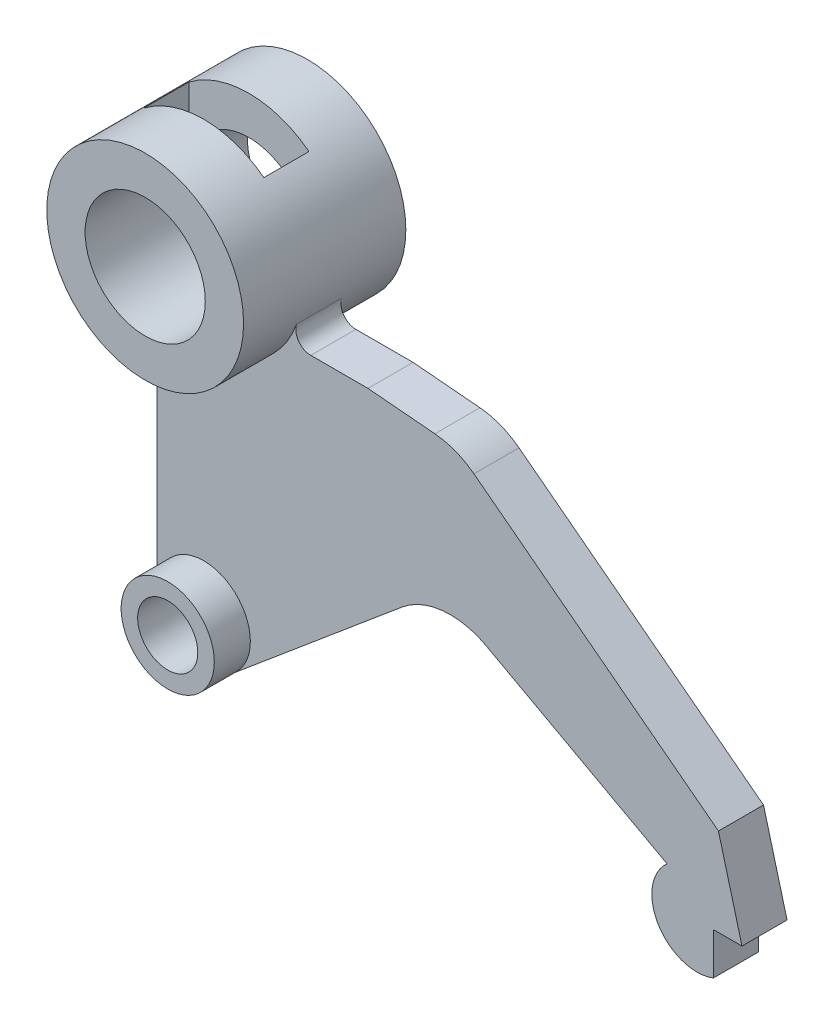
ISO-10303-21;
HEADER;
FILE_DESCRIPTION(('STEP AP214'),'2;1');
FILE_NAME('part.step','',(''),(''),'','','');
FILE_SCHEMA(('AUTOMOTIVE_DESIGN { 1 0 10303 214 1 1 1 1 }'));
ENDSEC;
DATA;
#1=APPLICATION_CONTEXT('core data for automotive mechanical design processes');
#2=APPLICATION_PROTOCOL_DEFINITION('international standard','automotive_design',2000,#1);
#3=PRODUCT_CONTEXT('',#1,'mechanical');
#4=PRODUCT('Part','Part','',(#3));
#5=PRODUCT_RELATED_PRODUCT_CATEGORY('part','',(#4));
#6=PRODUCT_DEFINITION_FORMATION('','',#4);
#7=PRODUCT_DEFINITION_CONTEXT('part definition',#1,'design');
#8=PRODUCT_DEFINITION('design','',#6,#7);
#9=PRODUCT_DEFINITION_SHAPE('','',#8);
#10=(LENGTH_UNIT() NAMED_UNIT(*) SI_UNIT(.MILLI.,.METRE.));
#11=(NAMED_UNIT(*) PLANE_ANGLE_UNIT() SI_UNIT($,.RADIAN.));
#12=(NAMED_UNIT(*) SI_UNIT($,.STERADIAN.) SOLID_ANGLE_UNIT());
#13=UNCERTAINTY_MEASURE_WITH_UNIT(LENGTH_MEASURE(1.E-05),#10,'distance_accuracy_value','');
#14=(GEOMETRIC_REPRESENTATION_CONTEXT(3) GLOBAL_UNCERTAINTY_ASSIGNED_CONTEXT((#13)) GLOBAL_UNIT_ASSIGNED_CONTEXT((#10,
#11,#12)) REPRESENTATION_CONTEXT('',''));
#15=CARTESIAN_POINT('',(0.,0.,0.));
#16=DIRECTION('',(0.,0.,1.));
#17=DIRECTION('',(1.,0.,0.));
#18=AXIS2_PLACEMENT_3D('',#15,#16,#17);
#19=CARTESIAN_POINT('',(0.,0.,16.2));
#20=DIRECTION('',(0.,0.,-1.));
#21=DIRECTION('',(-1.,0.,0.));
#22=AXIS2_PLACEMENT_3D('',#19,#20,#21);
#23=CYLINDRICAL_SURFACE('',#22,19.65);
#24=DIRECTION('',(0.,0.,-1.));
#25=VECTOR('',#24,1.);
#26=CARTESIAN_POINT('',(12.,15.560285987089,16.2));
#27=LINE('',#26,#25);
#28=CARTESIAN_POINT('',(12.,15.560285987089,-4.5));
#29=VERTEX_POINT('',#28);
#30=CARTESIAN_POINT('',(12.,15.560285987089,4.5));
#31=VERTEX_POINT('',#30);
#32=EDGE_CURVE('E11',#29,#31,#27,.F.);
#33=ORIENTED_EDGE('',*,*,#32,.T.);
#34=CARTESIAN_POINT('',(0.,0.,4.5));
#35=DIRECTION('',(0.,0.,1.));
#36=DIRECTION('',(1.,0.,0.));
#37=AXIS2_PLACEMENT_3D('',#34,#35,#36);
#38=CIRCLE('',#37,19.65);
#39=CARTESIAN_POINT('',(-12.,15.5602859870891,4.5));
#40=VERTEX_POINT('',#39);
#41=EDGE_CURVE('E53',#31,#40,#38,.T.);
#42=ORIENTED_EDGE('',*,*,#41,.T.);
#43=DIRECTION('',(0.,0.,-1.));
#44=VECTOR('',#43,1.);
#45=CARTESIAN_POINT('',(-12.,15.5602859870891,16.2));
#46=LINE('',#45,#44);
#47=CARTESIAN_POINT('',(-12.,15.5602859870891,-4.5));
#48=VERTEX_POINT('',#47);
#49=EDGE_CURVE('E48',#40,#48,#46,.T.);
#50=ORIENTED_EDGE('',*,*,#49,.T.);
#51=CARTESIAN_POINT('',(0.,0.,-4.5));
#52=DIRECTION('',(0.,0.,-1.));
#53=DIRECTION('',(-1.,0.,0.));
#54=AXIS2_PLACEMENT_3D('',#51,#52,#53);
#55=CIRCLE('',#54,19.65);
#56=EDGE_CURVE('E224',#48,#29,#55,.T.);
#57=ORIENTED_EDGE('',*,*,#56,.T.);
#58=EDGE_LOOP('',(#33,#42,#50,#57));
#59=FACE_BOUND('',#58,.T.);
#60=DIRECTION('',(0.,0.,-1.));
#61=VECTOR('',#60,1.);
#62=CARTESIAN_POINT('',(-13.7805194805195,-14.0078471881665,4.5));
#63=LINE('',#62,#61);
#64=CARTESIAN_POINT('',(-13.7805194805195,-14.0078471881665,4.5));
#65=VERTEX_POINT('',#64);
#66=CARTESIAN_POINT('',(-13.7805194805195,-14.0078471881665,-4.5));
#67=VERTEX_POINT('',#66);
#68=EDGE_CURVE('E360',#65,#67,#63,.T.);
#69=ORIENTED_EDGE('',*,*,#68,.F.);
#70=CARTESIAN_POINT('',(0.,0.,4.5));
#71=DIRECTION('',(0.,0.,1.));
#72=DIRECTION('',(1.,0.,0.));
#73=AXIS2_PLACEMENT_3D('',#70,#71,#72);
#74=CIRCLE('',#73,19.65);
#75=CARTESIAN_POINT('',(18.5414768405066,-6.50662251655629,4.5));
#76=VERTEX_POINT('',#75);
#77=EDGE_CURVE('E249',#65,#76,#74,.T.);
#78=ORIENTED_EDGE('',*,*,#77,.T.);
#79=DIRECTION('',(0.,0.,-1.));
#80=VECTOR('',#79,1.);
#81=CARTESIAN_POINT('',(18.5414768405066,-6.50662251655629,4.5));
#82=LINE('',#81,#80);
#83=CARTESIAN_POINT('',(18.5414768405066,-6.50662251655629,-4.5));
#84=VERTEX_POINT('',#83);
#85=EDGE_CURVE('E365',#76,#84,#82,.T.);
#86=ORIENTED_EDGE('',*,*,#85,.T.);
#87=CARTESIAN_POINT('',(0.,0.,-4.5));
#88=DIRECTION('',(0.,0.,1.));
#89=DIRECTION('',(1.,0.,0.));
#90=AXIS2_PLACEMENT_3D('',#87,#88,#89);
#91=CIRCLE('',#90,19.65);
#92=EDGE_CURVE('E287',#67,#84,#91,.T.);
#93=ORIENTED_EDGE('',*,*,#92,.F.);
#94=EDGE_LOOP('',(#69,#78,#86,#93));
#95=FACE_BOUND('',#94,.T.);
#96=CARTESIAN_POINT('',(0.,0.,16.2));
#97=DIRECTION('',(0.,0.,1.));
#98=DIRECTION('',(1.,0.,0.));
#99=AXIS2_PLACEMENT_3D('',#96,#97,#98);
#100=CIRCLE('',#99,19.65);
#101=CARTESIAN_POINT('',(19.65,0.,16.2));
#102=VERTEX_POINT('',#101);
#103=EDGE_CURVE('E362',#102,#102,#100,.T.);
#104=ORIENTED_EDGE('',*,*,#103,.F.);
#105=EDGE_LOOP('',(#104));
#106=FACE_BOUND('',#105,.T.);
#107=CARTESIAN_POINT('',(0.,0.,-16.2));
#108=DIRECTION('',(0.,0.,1.));
#109=DIRECTION('',(1.,0.,0.));
#110=AXIS2_PLACEMENT_3D('',#107,#108,#109);
#111=CIRCLE('',#110,19.65);
#112=CARTESIAN_POINT('',(19.65,0.,-16.2));
#113=VERTEX_POINT('',#112);
#114=EDGE_CURVE('E364',#113,#113,#111,.T.);
#115=ORIENTED_EDGE('',*,*,#114,.T.);
#116=EDGE_LOOP('',(#115));
#117=FACE_BOUND('',#116,.T.);
#118=ADVANCED_FACE('F41',(#59,#95,#106,#117),#23,.T.);
#119=CARTESIAN_POINT('',(0.,0.,16.2));
#120=DIRECTION('',(0.,0.,1.));
#121=DIRECTION('',(1.,0.,0.));
#122=AXIS2_PLACEMENT_3D('',#119,#120,#121);
#123=PLANE('',#122);
#124=CARTESIAN_POINT('',(0.,0.,16.2));
#125=DIRECTION('',(0.,0.,1.));
#126=DIRECTION('',(1.,0.,0.));
#127=AXIS2_PLACEMENT_3D('',#124,#125,#126);
#128=CIRCLE('',#127,12.);
#129=CARTESIAN_POINT('',(12.,0.,16.2));
#130=VERTEX_POINT('',#129);
#131=EDGE_CURVE('E227',#130,#130,#128,.T.);
#132=ORIENTED_EDGE('',*,*,#131,.F.);
#133=EDGE_LOOP('',(#132));
#134=FACE_BOUND('',#133,.T.);
#135=ORIENTED_EDGE('',*,*,#103,.T.);
#136=EDGE_LOOP('',(#135));
#137=FACE_BOUND('',#136,.T.);
#138=ADVANCED_FACE('F407',(#134,#137),#123,.T.);
#139=CARTESIAN_POINT('',(0.,0.,-16.2));
#140=DIRECTION('',(0.,0.,1.));
#141=DIRECTION('',(1.,0.,0.));
#142=AXIS2_PLACEMENT_3D('',#139,#140,#141);
#143=PLANE('',#142);
#144=CARTESIAN_POINT('',(0.,0.,-16.2));
#145=DIRECTION('',(0.,0.,1.));
#146=DIRECTION('',(1.,0.,0.));
#147=AXIS2_PLACEMENT_3D('',#144,#145,#146);
#148=CIRCLE('',#147,12.);
#149=CARTESIAN_POINT('',(12.,0.,-16.2));
#150=VERTEX_POINT('',#149);
#151=EDGE_CURVE('E229',#150,#150,#148,.T.);
#152=ORIENTED_EDGE('',*,*,#151,.T.);
#153=EDGE_LOOP('',(#152));
#154=FACE_BOUND('',#153,.T.);
#155=ORIENTED_EDGE('',*,*,#114,.F.);
#156=EDGE_LOOP('',(#155));
#157=FACE_BOUND('',#156,.T.);
#158=ADVANCED_FACE('F405',(#154,#157),#143,.F.);
#159=CARTESIAN_POINT('',(21.3722366634847,-7.5,4.5));
#160=DIRECTION('',(0.,0.,-1.));
#161=DIRECTION('',(-1.,0.,0.));
#162=AXIS2_PLACEMENT_3D('',#159,#160,#161);
#163=CYLINDRICAL_SURFACE('',#162,3.);
#164=CARTESIAN_POINT('',(21.3722366634847,-7.5,-4.5));
#165=DIRECTION('',(0.,0.,1.));
#166=DIRECTION('',(1.,0.,0.));
#167=AXIS2_PLACEMENT_3D('',#164,#165,#166);
#168=CIRCLE('',#167,3.);
#169=CARTESIAN_POINT('',(21.3722366634847,-10.5,-4.5));
#170=VERTEX_POINT('',#169);
#171=EDGE_CURVE('E246',#84,#170,#168,.T.);
#172=ORIENTED_EDGE('',*,*,#171,.F.);
#173=ORIENTED_EDGE('',*,*,#85,.F.);
#174=CARTESIAN_POINT('',(21.3722366634847,-7.5,4.5));
#175=DIRECTION('',(0.,0.,1.));
#176=DIRECTION('',(1.,0.,0.));
#177=AXIS2_PLACEMENT_3D('',#174,#175,#176);
#178=CIRCLE('',#177,3.);
#179=CARTESIAN_POINT('',(21.3722366634847,-10.5,4.5));
#180=VERTEX_POINT('',#179);
#181=EDGE_CURVE('E250',#76,#180,#178,.T.);
#182=ORIENTED_EDGE('',*,*,#181,.T.);
#183=DIRECTION('',(0.,0.,-1.));
#184=VECTOR('',#183,1.);
#185=CARTESIAN_POINT('',(21.3722366634847,-10.5,4.5));
#186=LINE('',#185,#184);
#187=EDGE_CURVE('E288',#180,#170,#186,.T.);
#188=ORIENTED_EDGE('',*,*,#187,.T.);
#189=EDGE_LOOP('',(#172,#173,#182,#188));
#190=FACE_BOUND('',#189,.T.);
#191=ADVANCED_FACE('F403',(#190),#163,.F.);
#192=CARTESIAN_POINT('',(-24.3,-24.7008603089042,4.5));
#193=DIRECTION('',(0.,0.,-1.));
#194=DIRECTION('',(-1.,0.,0.));
#195=AXIS2_PLACEMENT_3D('',#192,#193,#194);
#196=CYLINDRICAL_SURFACE('',#195,15.);
#197=CARTESIAN_POINT('',(-24.3,-24.7008603089042,-4.5));
#198=DIRECTION('',(0.,0.,1.));
#199=DIRECTION('',(1.,0.,0.));
#200=AXIS2_PLACEMENT_3D('',#197,#198,#199);
#201=CIRCLE('',#200,15.);
#202=CARTESIAN_POINT('',(-9.29999999999999,-24.7008603089042,-4.5));
#203=VERTEX_POINT('',#202);
#204=EDGE_CURVE('E292',#203,#67,#201,.T.);
#205=ORIENTED_EDGE('',*,*,#204,.F.);
#206=DIRECTION('',(0.,0.,-1.));
#207=VECTOR('',#206,1.);
#208=CARTESIAN_POINT('',(-9.29999999999999,-24.7008603089042,4.5));
#209=LINE('',#208,#207);
#210=CARTESIAN_POINT('',(-9.29999999999999,-24.7008603089042,4.5));
#211=VERTEX_POINT('',#210);
#212=EDGE_CURVE('E357',#211,#203,#209,.T.);
#213=ORIENTED_EDGE('',*,*,#212,.F.);
#214=CARTESIAN_POINT('',(-24.3,-24.7008603089042,4.5));
#215=DIRECTION('',(0.,0.,1.));
#216=DIRECTION('',(1.,0.,0.));
#217=AXIS2_PLACEMENT_3D('',#214,#215,#216);
#218=CIRCLE('',#217,15.);
#219=EDGE_CURVE('E254',#211,#65,#218,.T.);
#220=ORIENTED_EDGE('',*,*,#219,.T.);
#221=ORIENTED_EDGE('',*,*,#68,.T.);
#222=EDGE_LOOP('',(#205,#213,#220,#221));
#223=FACE_BOUND('',#222,.T.);
#224=ADVANCED_FACE('F422',(#223),#196,.F.);
#225=CARTESIAN_POINT('',(-9.29999999999999,0.,4.5));
#226=DIRECTION('',(-1.,0.,0.));
#227=DIRECTION('',(0.,0.,1.));
#228=AXIS2_PLACEMENT_3D('',#225,#226,#227);
#229=PLANE('',#228);
#230=DIRECTION('',(0.,1.,0.));
#231=VECTOR('',#230,1.);
#232=CARTESIAN_POINT('',(-9.29999999999999,0.,-4.5));
#233=LINE('',#232,#231);
#234=CARTESIAN_POINT('',(-9.29999999999999,-66.,-4.5));
#235=VERTEX_POINT('',#234);
#236=EDGE_CURVE('E294',#235,#203,#233,.T.);
#237=ORIENTED_EDGE('',*,*,#236,.F.);
#238=DIRECTION('',(0.,0.,-1.));
#239=VECTOR('',#238,1.);
#240=CARTESIAN_POINT('',(-9.29999999999999,-66.,4.5));
#241=LINE('',#240,#239);
#242=CARTESIAN_POINT('',(-9.29999999999999,-66.,4.5));
#243=VERTEX_POINT('',#242);
#244=EDGE_CURVE('E352',#243,#235,#241,.T.);
#245=ORIENTED_EDGE('',*,*,#244,.F.);
#246=DIRECTION('',(0.,1.,0.));
#247=VECTOR('',#246,1.);
#248=CARTESIAN_POINT('',(-9.29999999999999,0.,4.5));
#249=LINE('',#248,#247);
#250=EDGE_CURVE('E257',#243,#211,#249,.T.);
#251=ORIENTED_EDGE('',*,*,#250,.T.);
#252=ORIENTED_EDGE('',*,*,#212,.T.);
#253=EDGE_LOOP('',(#237,#245,#251,#252));
#254=FACE_BOUND('',#253,.T.);
#255=ADVANCED_FACE('F428',(#254),#229,.T.);
#256=CARTESIAN_POINT('',(0.,-66.,4.5));
#257=DIRECTION('',(0.,0.,-1.));
#258=DIRECTION('',(-1.,0.,0.));
#259=AXIS2_PLACEMENT_3D('',#256,#257,#258);
#260=CYLINDRICAL_SURFACE('',#259,9.3);
#261=ORIENTED_EDGE('',*,*,#244,.T.);
#262=CARTESIAN_POINT('',(0.,-66.,-4.5));
#263=DIRECTION('',(0.,0.,1.));
#264=DIRECTION('',(1.,0.,0.));
#265=AXIS2_PLACEMENT_3D('',#262,#263,#264);
#266=CIRCLE('',#265,9.3);
#267=CARTESIAN_POINT('',(5.97792477008489,-73.1242133210065,-4.5));
#268=VERTEX_POINT('',#267);
#269=EDGE_CURVE('E368',#268,#235,#266,.T.);
#270=ORIENTED_EDGE('',*,*,#269,.F.);
#271=DIRECTION('',(0.,0.,-1.));
#272=VECTOR('',#271,1.);
#273=CARTESIAN_POINT('',(5.97792477008485,-73.1242133210065,4.5));
#274=LINE('',#273,#272);
#275=CARTESIAN_POINT('',(5.97792477008485,-73.1242133210065,4.5));
#276=VERTEX_POINT('',#275);
#277=EDGE_CURVE('E353',#276,#268,#274,.T.);
#278=ORIENTED_EDGE('',*,*,#277,.F.);
#279=CARTESIAN_POINT('',(0.,-66.,4.5));
#280=DIRECTION('',(0.,0.,1.));
#281=DIRECTION('',(1.,0.,0.));
#282=AXIS2_PLACEMENT_3D('',#279,#280,#281);
#283=CIRCLE('',#282,9.3);
#284=EDGE_CURVE('E243',#276,#243,#283,.T.);
#285=ORIENTED_EDGE('',*,*,#284,.T.);
#286=EDGE_LOOP('',(#261,#270,#278,#285));
#287=FACE_BOUND('',#286,.T.);
#288=CARTESIAN_POINT('',(0.,-66.,-11.7));
#289=DIRECTION('',(0.,0.,1.));
#290=DIRECTION('',(1.,0.,0.));
#291=AXIS2_PLACEMENT_3D('',#288,#289,#290);
#292=CIRCLE('',#291,9.3);
#293=CARTESIAN_POINT('',(9.30000000000001,-66.,-11.7));
#294=VERTEX_POINT('',#293);
#295=EDGE_CURVE('E239',#294,#294,#292,.T.);
#296=ORIENTED_EDGE('',*,*,#295,.T.);
#297=EDGE_LOOP('',(#296));
#298=FACE_BOUND('',#297,.T.);
#299=CARTESIAN_POINT('',(0.,-66.,11.7));
#300=DIRECTION('',(0.,0.,1.));
#301=DIRECTION('',(1.,0.,0.));
#302=AXIS2_PLACEMENT_3D('',#299,#300,#301);
#303=CIRCLE('',#302,9.3);
#304=CARTESIAN_POINT('',(9.30000000000001,-66.,11.7));
#305=VERTEX_POINT('',#304);
#306=EDGE_CURVE('E240',#305,#305,#303,.T.);
#307=ORIENTED_EDGE('',*,*,#306,.F.);
#308=EDGE_LOOP('',(#307));
#309=FACE_BOUND('',#308,.T.);
#310=ADVANCED_FACE('F427',(#287,#298,#309),#260,.T.);
#311=CARTESIAN_POINT('',(38.4765806194879,-45.8546031840146,4.5));
#312=DIRECTION('',(-0.642787609686546,0.766044443118972,0.));
#313=DIRECTION('',(-0.766044443118973,-0.642787609686546,0.));
#314=AXIS2_PLACEMENT_3D('',#311,#312,#313);
#315=PLANE('',#314);
#316=DIRECTION('',(0.766044443118972,0.642787609686546,0.));
#317=VECTOR('',#316,1.);
#318=CARTESIAN_POINT('',(38.4765806194879,-45.8546031840146,-4.5));
#319=LINE('',#318,#317);
#320=CARTESIAN_POINT('',(39.5950196885321,-44.9161213736853,-4.5));
#321=VERTEX_POINT('',#320);
#322=EDGE_CURVE('E296',#268,#321,#319,.T.);
#323=ORIENTED_EDGE('',*,*,#322,.T.);
#324=DIRECTION('',(0.,0.,-1.));
#325=VECTOR('',#324,1.);
#326=CARTESIAN_POINT('',(39.5950196885321,-44.9161213736853,4.5));
#327=LINE('',#326,#325);
#328=CARTESIAN_POINT('',(39.5950196885321,-44.9161213736853,4.5));
#329=VERTEX_POINT('',#328);
#330=EDGE_CURVE('E346',#329,#321,#327,.T.);
#331=ORIENTED_EDGE('',*,*,#330,.F.);
#332=DIRECTION('',(0.766044443118972,0.642787609686546,0.));
#333=VECTOR('',#332,1.);
#334=CARTESIAN_POINT('',(38.4765806194879,-45.8546031840146,4.5));
#335=LINE('',#334,#333);
#336=EDGE_CURVE('E256',#276,#329,#335,.T.);
#337=ORIENTED_EDGE('',*,*,#336,.F.);
#338=ORIENTED_EDGE('',*,*,#277,.T.);
#339=EDGE_LOOP('',(#323,#331,#337,#338));
#340=FACE_BOUND('',#339,.T.);
#341=ADVANCED_FACE('F432',(#340),#315,.F.);
#342=CARTESIAN_POINT('',(49.2368338338303,-56.4067880204702,4.5));
#343=DIRECTION('',(0.,0.,-1.));
#344=DIRECTION('',(-1.,0.,0.));
#345=AXIS2_PLACEMENT_3D('',#342,#343,#344);
#346=CYLINDRICAL_SURFACE('',#345,15.0000000000003);
#347=CARTESIAN_POINT('',(49.2368338338303,-56.4067880204702,-4.5));
#348=DIRECTION('',(0.,0.,1.));
#349=DIRECTION('',(1.,0.,0.));
#350=AXIS2_PLACEMENT_3D('',#347,#348,#349);
#351=CIRCLE('',#350,15.0000000000003);
#352=CARTESIAN_POINT('',(56.4010062616653,-43.228220821254,-4.5));
#353=VERTEX_POINT('',#352);
#354=EDGE_CURVE('E301',#353,#321,#351,.T.);
#355=ORIENTED_EDGE('',*,*,#354,.F.);
#356=DIRECTION('',(0.,0.,-1.));
#357=VECTOR('',#356,1.);
#358=CARTESIAN_POINT('',(56.4010062616653,-43.228220821254,4.5));
#359=LINE('',#358,#357);
#360=CARTESIAN_POINT('',(56.4010062616653,-43.228220821254,4.5));
#361=VERTEX_POINT('',#360);
#362=EDGE_CURVE('E350',#361,#353,#359,.T.);
#363=ORIENTED_EDGE('',*,*,#362,.F.);
#364=CARTESIAN_POINT('',(49.2368338338303,-56.4067880204702,4.5));
#365=DIRECTION('',(0.,0.,1.));
#366=DIRECTION('',(1.,0.,0.));
#367=AXIS2_PLACEMENT_3D('',#364,#365,#366);
#368=CIRCLE('',#367,15.0000000000003);
#369=EDGE_CURVE('E262',#361,#329,#368,.T.);
#370=ORIENTED_EDGE('',*,*,#369,.T.);
#371=ORIENTED_EDGE('',*,*,#330,.T.);
#372=EDGE_LOOP('',(#355,#363,#370,#371));
#373=FACE_BOUND('',#372,.T.);
#374=ADVANCED_FACE('F438',(#373),#346,.F.);
#375=CARTESIAN_POINT('',(-5.27345113423973,-9.70056637307379,4.5));
#376=DIRECTION('',(0.477611495189005,0.87857114661439,0.));
#377=DIRECTION('',(-0.87857114661439,0.477611495189005,0.));
#378=AXIS2_PLACEMENT_3D('',#375,#376,#377);
#379=PLANE('',#378);
#380=DIRECTION('',(0.87857114661439,-0.477611495189005,0.));
#381=VECTOR('',#380,1.);
#382=CARTESIAN_POINT('',(-5.27345113423973,-9.70056637307379,-4.5));
#383=LINE('',#382,#381);
#384=CARTESIAN_POINT('',(92.5111026573235,-62.8585002783132,-4.5));
#385=VERTEX_POINT('',#384);
#386=EDGE_CURVE('E302',#353,#385,#383,.T.);
#387=ORIENTED_EDGE('',*,*,#386,.T.);
#388=DIRECTION('',(0.,0.,-1.));
#389=VECTOR('',#388,1.);
#390=CARTESIAN_POINT('',(92.5111026573235,-62.8585002783132,4.5));
#391=LINE('',#390,#389);
#392=CARTESIAN_POINT('',(92.5111026573235,-62.8585002783132,4.5));
#393=VERTEX_POINT('',#392);
#394=EDGE_CURVE('E341',#393,#385,#391,.T.);
#395=ORIENTED_EDGE('',*,*,#394,.F.);
#396=DIRECTION('',(0.87857114661439,-0.477611495189005,0.));
#397=VECTOR('',#396,1.);
#398=CARTESIAN_POINT('',(-5.27345113423973,-9.70056637307379,4.5));
#399=LINE('',#398,#397);
#400=EDGE_CURVE('E261',#361,#393,#399,.T.);
#401=ORIENTED_EDGE('',*,*,#400,.F.);
#402=ORIENTED_EDGE('',*,*,#362,.T.);
#403=EDGE_LOOP('',(#387,#395,#401,#402));
#404=FACE_BOUND('',#403,.T.);
#405=ADVANCED_FACE('F445',(#404),#379,.F.);
#406=CARTESIAN_POINT('',(98.4736676676606,-69.6,4.5));
#407=DIRECTION('',(0.,0.,-1.));
#408=DIRECTION('',(-1.,0.,0.));
#409=AXIS2_PLACEMENT_3D('',#406,#407,#408);
#410=CYLINDRICAL_SURFACE('',#409,9.);
#411=CARTESIAN_POINT('',(98.4736676676606,-69.6,-4.5));
#412=DIRECTION('',(0.,0.,1.));
#413=DIRECTION('',(1.,0.,0.));
#414=AXIS2_PLACEMENT_3D('',#411,#412,#413);
#415=CIRCLE('',#414,9.);
#416=CARTESIAN_POINT('',(101.773667667661,-77.9731714421717,-4.5));
#417=VERTEX_POINT('',#416);
#418=EDGE_CURVE('E306',#385,#417,#415,.T.);
#419=ORIENTED_EDGE('',*,*,#418,.T.);
#420=DIRECTION('',(0.,0.,-1.));
#421=VECTOR('',#420,1.);
#422=CARTESIAN_POINT('',(101.773667667661,-77.9731714421717,4.5));
#423=LINE('',#422,#421);
#424=CARTESIAN_POINT('',(101.773667667661,-77.9731714421717,4.5));
#425=VERTEX_POINT('',#424);
#426=EDGE_CURVE('E342',#425,#417,#423,.T.);
#427=ORIENTED_EDGE('',*,*,#426,.F.);
#428=CARTESIAN_POINT('',(98.4736676676606,-69.6,4.5));
#429=DIRECTION('',(0.,0.,1.));
#430=DIRECTION('',(1.,0.,0.));
#431=AXIS2_PLACEMENT_3D('',#428,#429,#430);
#432=CIRCLE('',#431,9.);
#433=EDGE_CURVE('E268',#393,#425,#432,.T.);
#434=ORIENTED_EDGE('',*,*,#433,.F.);
#435=ORIENTED_EDGE('',*,*,#394,.T.);
#436=EDGE_LOOP('',(#419,#427,#434,#435));
#437=FACE_BOUND('',#436,.T.);
#438=ADVANCED_FACE('F447',(#437),#410,.T.);
#439=CARTESIAN_POINT('',(101.773667667661,0.,4.5));
#440=DIRECTION('',(-1.,0.,0.));
#441=DIRECTION('',(0.,0.,1.));
#442=AXIS2_PLACEMENT_3D('',#439,#440,#441);
#443=PLANE('',#442);
#444=DIRECTION('',(0.,1.,0.));
#445=VECTOR('',#444,1.);
#446=CARTESIAN_POINT('',(101.773667667661,0.,-4.5));
#447=LINE('',#446,#445);
#448=CARTESIAN_POINT('',(101.773667667661,-69.6,-4.5));
#449=VERTEX_POINT('',#448);
#450=EDGE_CURVE('E308',#417,#449,#447,.T.);
#451=ORIENTED_EDGE('',*,*,#450,.T.);
#452=DIRECTION('',(0.,0.,-1.));
#453=VECTOR('',#452,1.);
#454=CARTESIAN_POINT('',(101.773667667661,-69.6,4.5));
#455=LINE('',#454,#453);
#456=CARTESIAN_POINT('',(101.773667667661,-69.6,4.5));
#457=VERTEX_POINT('',#456);
#458=EDGE_CURVE('E336',#457,#449,#455,.T.);
#459=ORIENTED_EDGE('',*,*,#458,.F.);
#460=DIRECTION('',(0.,1.,0.));
#461=VECTOR('',#460,1.);
#462=CARTESIAN_POINT('',(101.773667667661,0.,4.5));
#463=LINE('',#462,#461);
#464=EDGE_CURVE('E266',#425,#457,#463,.T.);
#465=ORIENTED_EDGE('',*,*,#464,.F.);
#466=ORIENTED_EDGE('',*,*,#426,.T.);
#467=EDGE_LOOP('',(#451,#459,#465,#466));
#468=FACE_BOUND('',#467,.T.);
#469=ADVANCED_FACE('F448',(#468),#443,.F.);
#470=CARTESIAN_POINT('',(0.,-69.6,4.5));
#471=DIRECTION('',(0.,1.,0.));
#472=DIRECTION('',(0.,0.,1.));
#473=AXIS2_PLACEMENT_3D('',#470,#471,#472);
#474=PLANE('',#473);
#475=DIRECTION('',(1.,0.,0.));
#476=VECTOR('',#475,1.);
#477=CARTESIAN_POINT('',(0.,-69.6,-4.5));
#478=LINE('',#477,#476);
#479=CARTESIAN_POINT('',(107.473667667661,-69.6,-4.5));
#480=VERTEX_POINT('',#479);
#481=EDGE_CURVE('E309',#449,#480,#478,.T.);
#482=ORIENTED_EDGE('',*,*,#481,.T.);
#483=DIRECTION('',(0.,0.,-1.));
#484=VECTOR('',#483,1.);
#485=CARTESIAN_POINT('',(107.473667667661,-69.6,4.5));
#486=LINE('',#485,#484);
#487=CARTESIAN_POINT('',(107.473667667661,-69.6,4.5));
#488=VERTEX_POINT('',#487);
#489=EDGE_CURVE('E334',#488,#480,#486,.T.);
#490=ORIENTED_EDGE('',*,*,#489,.F.);
#491=DIRECTION('',(1.,0.,0.));
#492=VECTOR('',#491,1.);
#493=CARTESIAN_POINT('',(0.,-69.6,4.5));
#494=LINE('',#493,#492);
#495=EDGE_CURVE('E269',#457,#488,#494,.T.);
#496=ORIENTED_EDGE('',*,*,#495,.F.);
#497=ORIENTED_EDGE('',*,*,#458,.T.);
#498=EDGE_LOOP('',(#482,#490,#496,#497));
#499=FACE_BOUND('',#498,.T.);
#500=ADVANCED_FACE('F451',(#499),#474,.F.);
#501=CARTESIAN_POINT('',(82.8742970528694,22.2061009686142,4.5));
#502=DIRECTION('',(-0.965925826289066,-0.25881904510253,0.));
#503=DIRECTION('',(0.25881904510253,-0.965925826289066,0.));
#504=AXIS2_PLACEMENT_3D('',#501,#502,#503);
#505=PLANE('',#504);
#506=DIRECTION('',(-0.25881904510253,0.965925826289066,0.));
#507=VECTOR('',#506,1.);
#508=CARTESIAN_POINT('',(82.8742970528694,22.2061009686142,-4.5));
#509=LINE('',#508,#507);
#510=CARTESIAN_POINT('',(102.772365266735,-52.0545005780013,-4.5));
#511=VERTEX_POINT('',#510);
#512=EDGE_CURVE('E315',#480,#511,#509,.T.);
#513=ORIENTED_EDGE('',*,*,#512,.T.);
#514=DIRECTION('',(0.,0.,-1.));
#515=VECTOR('',#514,1.);
#516=CARTESIAN_POINT('',(102.772365266735,-52.0545005780013,4.5));
#517=LINE('',#516,#515);
#518=CARTESIAN_POINT('',(102.772365266735,-52.0545005780013,4.5));
#519=VERTEX_POINT('',#518);
#520=EDGE_CURVE('E331',#519,#511,#517,.T.);
#521=ORIENTED_EDGE('',*,*,#520,.F.);
#522=DIRECTION('',(-0.25881904510253,0.965925826289066,0.));
#523=VECTOR('',#522,1.);
#524=CARTESIAN_POINT('',(82.8742970528694,22.2061009686142,4.5));
#525=LINE('',#524,#523);
#526=EDGE_CURVE('E275',#488,#519,#525,.T.);
#527=ORIENTED_EDGE('',*,*,#526,.F.);
#528=ORIENTED_EDGE('',*,*,#489,.T.);
#529=EDGE_LOOP('',(#513,#521,#527,#528));
#530=FACE_BOUND('',#529,.T.);
#531=ADVANCED_FACE('F459',(#530),#505,.F.);
#532=CARTESIAN_POINT('',(12.8288470120228,16.7663169030326,4.5));
#533=DIRECTION('',(0.607675623707297,0.794185328718648,0.));
#534=DIRECTION('',(-0.794185328718648,0.607675623707297,0.));
#535=AXIS2_PLACEMENT_3D('',#532,#533,#534);
#536=PLANE('',#535);
#537=DIRECTION('',(0.794185328718648,-0.607675623707297,0.));
#538=VECTOR('',#537,1.);
#539=CARTESIAN_POINT('',(12.8288470120228,16.7663169030326,-4.5));
#540=LINE('',#539,#538);
#541=CARTESIAN_POINT('',(53.950427647652,-14.698104884893,-4.5));
#542=VERTEX_POINT('',#541);
#543=EDGE_CURVE('E314',#542,#511,#540,.T.);
#544=ORIENTED_EDGE('',*,*,#543,.F.);
#545=DIRECTION('',(0.,0.,-1.));
#546=VECTOR('',#545,1.);
#547=CARTESIAN_POINT('',(53.950427647652,-14.698104884893,4.5));
#548=LINE('',#547,#546);
#549=CARTESIAN_POINT('',(53.950427647652,-14.698104884893,4.5));
#550=VERTEX_POINT('',#549);
#551=EDGE_CURVE('E333',#550,#542,#548,.T.);
#552=ORIENTED_EDGE('',*,*,#551,.F.);
#553=DIRECTION('',(0.794185328718648,-0.607675623707297,0.));
#554=VECTOR('',#553,1.);
#555=CARTESIAN_POINT('',(12.8288470120228,16.7663169030326,4.5));
#556=LINE('',#555,#554);
#557=EDGE_CURVE('E274',#550,#519,#556,.T.);
#558=ORIENTED_EDGE('',*,*,#557,.T.);
#559=ORIENTED_EDGE('',*,*,#520,.T.);
#560=EDGE_LOOP('',(#544,#552,#558,#559));
#561=FACE_BOUND('',#560,.T.);
#562=ADVANCED_FACE('F465',(#561),#536,.T.);
#563=CARTESIAN_POINT('',(44.8352932920425,-26.6108848156727,4.5));
#564=DIRECTION('',(0.,0.,-1.));
#565=DIRECTION('',(-1.,0.,0.));
#566=AXIS2_PLACEMENT_3D('',#563,#564,#565);
#567=CYLINDRICAL_SURFACE('',#566,15.);
#568=CARTESIAN_POINT('',(44.8352932920425,-26.6108848156727,-4.5));
#569=DIRECTION('',(0.,0.,1.));
#570=DIRECTION('',(1.,0.,0.));
#571=AXIS2_PLACEMENT_3D('',#568,#569,#570);
#572=CIRCLE('',#571,15.);
#573=CARTESIAN_POINT('',(46.1426294332573,-11.6679643442965,-4.5));
#574=VERTEX_POINT('',#573);
#575=EDGE_CURVE('E319',#574,#542,#572,.F.);
#576=ORIENTED_EDGE('',*,*,#575,.F.);
#577=DIRECTION('',(0.,0.,-1.));
#578=VECTOR('',#577,1.);
#579=CARTESIAN_POINT('',(46.1426294332573,-11.6679643442965,4.5));
#580=LINE('',#579,#578);
#581=CARTESIAN_POINT('',(46.1426294332573,-11.6679643442965,4.5));
#582=VERTEX_POINT('',#581);
#583=EDGE_CURVE('E326',#582,#574,#580,.T.);
#584=ORIENTED_EDGE('',*,*,#583,.F.);
#585=CARTESIAN_POINT('',(44.8352932920425,-26.6108848156727,4.5));
#586=DIRECTION('',(0.,0.,1.));
#587=DIRECTION('',(1.,0.,0.));
#588=AXIS2_PLACEMENT_3D('',#585,#586,#587);
#589=CIRCLE('',#588,15.);
#590=EDGE_CURVE('E280',#582,#550,#589,.F.);
#591=ORIENTED_EDGE('',*,*,#590,.T.);
#592=ORIENTED_EDGE('',*,*,#551,.T.);
#593=EDGE_LOOP('',(#576,#584,#591,#592));
#594=FACE_BOUND('',#593,.T.);
#595=ADVANCED_FACE('F467',(#594),#567,.T.);
#596=CARTESIAN_POINT('',(-0.662555261226807,-7.57304128929202,4.5));
#597=DIRECTION('',(0.0871557427476592,0.996194698091745,0.));
#598=DIRECTION('',(-0.996194698091746,0.0871557427476592,0.));
#599=AXIS2_PLACEMENT_3D('',#596,#597,#598);
#600=PLANE('',#599);
#601=DIRECTION('',(0.996194698091745,-0.0871557427476592,0.));
#602=VECTOR('',#601,1.);
#603=CARTESIAN_POINT('',(-0.662555261226807,-7.57304128929202,-4.5));
#604=LINE('',#603,#602);
#605=CARTESIAN_POINT('',(32.7927358901879,-10.5,-4.5));
#606=VERTEX_POINT('',#605);
#607=EDGE_CURVE('E322',#606,#574,#604,.T.);
#608=ORIENTED_EDGE('',*,*,#607,.F.);
#609=DIRECTION('',(0.,0.,-1.));
#610=VECTOR('',#609,1.);
#611=CARTESIAN_POINT('',(32.7927358901879,-10.5,4.5));
#612=LINE('',#611,#610);
#613=CARTESIAN_POINT('',(32.7927358901879,-10.5,4.5));
#614=VERTEX_POINT('',#613);
#615=EDGE_CURVE('E330',#614,#606,#612,.T.);
#616=ORIENTED_EDGE('',*,*,#615,.F.);
#617=DIRECTION('',(0.996194698091745,-0.0871557427476592,0.));
#618=VECTOR('',#617,1.);
#619=CARTESIAN_POINT('',(-0.662555261226807,-7.57304128929202,4.5));
#620=LINE('',#619,#618);
#621=EDGE_CURVE('E278',#614,#582,#620,.T.);
#622=ORIENTED_EDGE('',*,*,#621,.T.);
#623=ORIENTED_EDGE('',*,*,#583,.T.);
#624=EDGE_LOOP('',(#608,#616,#622,#623));
#625=FACE_BOUND('',#624,.T.);
#626=ADVANCED_FACE('F468',(#625),#600,.T.);
#627=CARTESIAN_POINT('',(0.,-10.5,4.5));
#628=DIRECTION('',(0.,1.,0.));
#629=DIRECTION('',(0.,0.,1.));
#630=AXIS2_PLACEMENT_3D('',#627,#628,#629);
#631=PLANE('',#630);
#632=DIRECTION('',(1.,0.,0.));
#633=VECTOR('',#632,1.);
#634=CARTESIAN_POINT('',(0.,-10.5,-4.5));
#635=LINE('',#634,#633);
#636=EDGE_CURVE('E252',#170,#606,#635,.T.);
#637=ORIENTED_EDGE('',*,*,#636,.F.);
#638=ORIENTED_EDGE('',*,*,#187,.F.);
#639=DIRECTION('',(1.,0.,0.));
#640=VECTOR('',#639,1.);
#641=CARTESIAN_POINT('',(0.,-10.5,4.5));
#642=LINE('',#641,#640);
#643=EDGE_CURVE('E284',#180,#614,#642,.T.);
#644=ORIENTED_EDGE('',*,*,#643,.T.);
#645=ORIENTED_EDGE('',*,*,#615,.T.);
#646=EDGE_LOOP('',(#637,#638,#644,#645));
#647=FACE_BOUND('',#646,.T.);
#648=ADVANCED_FACE('F471',(#647),#631,.T.);
#649=CARTESIAN_POINT('',(0.,0.,4.5));
#650=DIRECTION('',(0.,0.,1.));
#651=DIRECTION('',(1.,0.,0.));
#652=AXIS2_PLACEMENT_3D('',#649,#650,#651);
#653=PLANE('',#652);
#654=ORIENTED_EDGE('',*,*,#284,.F.);
#655=ORIENTED_EDGE('',*,*,#336,.T.);
#656=ORIENTED_EDGE('',*,*,#369,.F.);
#657=ORIENTED_EDGE('',*,*,#400,.T.);
#658=ORIENTED_EDGE('',*,*,#433,.T.);
#659=ORIENTED_EDGE('',*,*,#464,.T.);
#660=ORIENTED_EDGE('',*,*,#495,.T.);
#661=ORIENTED_EDGE('',*,*,#526,.T.);
#662=ORIENTED_EDGE('',*,*,#557,.F.);
#663=ORIENTED_EDGE('',*,*,#590,.F.);
#664=ORIENTED_EDGE('',*,*,#621,.F.);
#665=ORIENTED_EDGE('',*,*,#643,.F.);
#666=ORIENTED_EDGE('',*,*,#181,.F.);
#667=ORIENTED_EDGE('',*,*,#77,.F.);
#668=ORIENTED_EDGE('',*,*,#219,.F.);
#669=ORIENTED_EDGE('',*,*,#250,.F.);
#670=EDGE_LOOP('',(#654,#655,#656,#657,#658,#659,#660,#661,#662,#663,#664,#665,#666,#667,#668,#669));
#671=FACE_BOUND('',#670,.T.);
#672=ADVANCED_FACE('F479',(#671),#653,.T.);
#673=CARTESIAN_POINT('',(0.,0.,-4.5));
#674=DIRECTION('',(0.,0.,1.));
#675=DIRECTION('',(1.,0.,0.));
#676=AXIS2_PLACEMENT_3D('',#673,#674,#675);
#677=PLANE('',#676);
#678=ORIENTED_EDGE('',*,*,#322,.F.);
#679=ORIENTED_EDGE('',*,*,#269,.T.);
#680=ORIENTED_EDGE('',*,*,#236,.T.);
#681=ORIENTED_EDGE('',*,*,#204,.T.);
#682=ORIENTED_EDGE('',*,*,#92,.T.);
#683=ORIENTED_EDGE('',*,*,#171,.T.);
#684=ORIENTED_EDGE('',*,*,#636,.T.);
#685=ORIENTED_EDGE('',*,*,#607,.T.);
#686=ORIENTED_EDGE('',*,*,#575,.T.);
#687=ORIENTED_EDGE('',*,*,#543,.T.);
#688=ORIENTED_EDGE('',*,*,#512,.F.);
#689=ORIENTED_EDGE('',*,*,#481,.F.);
#690=ORIENTED_EDGE('',*,*,#450,.F.);
#691=ORIENTED_EDGE('',*,*,#418,.F.);
#692=ORIENTED_EDGE('',*,*,#386,.F.);
#693=ORIENTED_EDGE('',*,*,#354,.T.);
#694=EDGE_LOOP('',(#678,#679,#680,#681,#682,#683,#684,#685,#686,#687,#688,#689,#690,#691,#692,#693));
#695=FACE_BOUND('',#694,.T.);
#696=ADVANCED_FACE('F478',(#695),#677,.F.);
#697=CARTESIAN_POINT('',(0.,-66.,-11.7));
#698=DIRECTION('',(0.,0.,1.));
#699=DIRECTION('',(1.,0.,0.));
#700=AXIS2_PLACEMENT_3D('',#697,#698,#699);
#701=PLANE('',#700);
#702=CARTESIAN_POINT('',(0.,-66.,-11.7));
#703=DIRECTION('',(0.,0.,1.));
#704=DIRECTION('',(1.,0.,0.));
#705=AXIS2_PLACEMENT_3D('',#702,#703,#704);
#706=CIRCLE('',#705,6.);
#707=CARTESIAN_POINT('',(6.00000000000001,-66.,-11.7));
#708=VERTEX_POINT('',#707);
#709=EDGE_CURVE('E234',#708,#708,#706,.T.);
#710=ORIENTED_EDGE('',*,*,#709,.T.);
#711=EDGE_LOOP('',(#710));
#712=FACE_BOUND('',#711,.T.);
#713=ORIENTED_EDGE('',*,*,#295,.F.);
#714=EDGE_LOOP('',(#713));
#715=FACE_BOUND('',#714,.T.);
#716=ADVANCED_FACE('F481',(#712,#715),#701,.F.);
#717=CARTESIAN_POINT('',(0.,-66.,11.7));
#718=DIRECTION('',(0.,0.,1.));
#719=DIRECTION('',(1.,0.,0.));
#720=AXIS2_PLACEMENT_3D('',#717,#718,#719);
#721=PLANE('',#720);
#722=CARTESIAN_POINT('',(0.,-66.,11.7));
#723=DIRECTION('',(0.,0.,1.));
#724=DIRECTION('',(1.,0.,0.));
#725=AXIS2_PLACEMENT_3D('',#722,#723,#724);
#726=CIRCLE('',#725,6.);
#727=CARTESIAN_POINT('',(6.00000000000001,-66.,11.7));
#728=VERTEX_POINT('',#727);
#729=EDGE_CURVE('E233',#728,#728,#726,.T.);
#730=ORIENTED_EDGE('',*,*,#729,.F.);
#731=EDGE_LOOP('',(#730));
#732=FACE_BOUND('',#731,.T.);
#733=ORIENTED_EDGE('',*,*,#306,.T.);
#734=EDGE_LOOP('',(#733));
#735=FACE_BOUND('',#734,.T.);
#736=ADVANCED_FACE('F489',(#732,#735),#721,.T.);
#737=CARTESIAN_POINT('',(0.,-66.,-28.5));
#738=DIRECTION('',(0.,0.,1.));
#739=DIRECTION('',(1.,0.,0.));
#740=AXIS2_PLACEMENT_3D('',#737,#738,#739);
#741=CYLINDRICAL_SURFACE('',#740,6.);
#742=CARTESIAN_POINT('',(6.00000000000001,-66.,11.7));
#743=CARTESIAN_POINT('',(6.00000000000001,-66.,11.45625));
#744=CARTESIAN_POINT('',(6.00000000000001,-66.,11.2125));
#745=CARTESIAN_POINT('',(6.00000000000001,-66.,10.725));
#746=CARTESIAN_POINT('',(6.00000000000001,-66.,10.48125));
#747=CARTESIAN_POINT('',(6.00000000000001,-66.,9.99375));
#748=CARTESIAN_POINT('',(6.00000000000001,-66.,9.75));
#749=CARTESIAN_POINT('',(6.00000000000001,-66.,9.2625));
#750=CARTESIAN_POINT('',(6.00000000000001,-66.,9.01875));
#751=CARTESIAN_POINT('',(6.00000000000001,-66.,8.53125));
#752=CARTESIAN_POINT('',(6.00000000000001,-66.,8.2875));
#753=CARTESIAN_POINT('',(6.00000000000001,-66.,7.8));
#754=CARTESIAN_POINT('',(6.00000000000001,-66.,7.55625));
#755=CARTESIAN_POINT('',(6.00000000000001,-66.,7.06875));
#756=CARTESIAN_POINT('',(6.00000000000001,-66.,6.825));
#757=CARTESIAN_POINT('',(6.00000000000001,-66.,6.3375));
#758=CARTESIAN_POINT('',(6.00000000000001,-66.,6.09375));
#759=CARTESIAN_POINT('',(6.00000000000001,-66.,5.60625));
#760=CARTESIAN_POINT('',(6.00000000000001,-66.,5.3625));
#761=CARTESIAN_POINT('',(6.00000000000001,-66.,4.875));
#762=CARTESIAN_POINT('',(6.00000000000001,-66.,4.63125));
#763=CARTESIAN_POINT('',(6.00000000000001,-66.,4.14375));
#764=CARTESIAN_POINT('',(6.00000000000001,-66.,3.9));
#765=CARTESIAN_POINT('',(6.00000000000001,-66.,3.4125));
#766=CARTESIAN_POINT('',(6.00000000000001,-66.,3.16874999999999));
#767=CARTESIAN_POINT('',(6.00000000000001,-66.,2.68125));
#768=CARTESIAN_POINT('',(6.00000000000001,-66.,2.4375));
#769=CARTESIAN_POINT('',(6.00000000000001,-66.,1.95));
#770=CARTESIAN_POINT('',(6.00000000000001,-66.,1.70625));
#771=CARTESIAN_POINT('',(6.00000000000001,-66.,1.21875));
#772=CARTESIAN_POINT('',(6.00000000000001,-66.,0.974999999999999));
#773=CARTESIAN_POINT('',(6.00000000000001,-66.,0.4875));
#774=CARTESIAN_POINT('',(6.00000000000001,-66.,0.24375));
#775=CARTESIAN_POINT('',(6.00000000000001,-66.,-0.24375));
#776=CARTESIAN_POINT('',(6.00000000000001,-66.,-0.4875));
#777=CARTESIAN_POINT('',(6.00000000000001,-66.,-0.974999999999999));
#778=CARTESIAN_POINT('',(6.00000000000001,-66.,-1.21875));
#779=CARTESIAN_POINT('',(6.00000000000001,-66.,-1.70625));
#780=CARTESIAN_POINT('',(6.00000000000001,-66.,-1.95));
#781=CARTESIAN_POINT('',(6.00000000000001,-66.,-2.4375));
#782=CARTESIAN_POINT('',(6.00000000000001,-66.,-2.68125));
#783=CARTESIAN_POINT('',(6.00000000000001,-66.,-3.16875));
#784=CARTESIAN_POINT('',(6.00000000000001,-66.,-3.4125));
#785=CARTESIAN_POINT('',(6.00000000000001,-66.,-3.9));
#786=CARTESIAN_POINT('',(6.00000000000001,-66.,-4.14375));
#787=CARTESIAN_POINT('',(6.00000000000001,-66.,-4.63125));
#788=CARTESIAN_POINT('',(6.00000000000001,-66.,-4.875));
#789=CARTESIAN_POINT('',(6.00000000000001,-66.,-5.3625));
#790=CARTESIAN_POINT('',(6.00000000000001,-66.,-5.60625));
#791=CARTESIAN_POINT('',(6.00000000000001,-66.,-6.09375));
#792=CARTESIAN_POINT('',(6.00000000000001,-66.,-6.3375));
#793=CARTESIAN_POINT('',(6.00000000000001,-66.,-6.825));
#794=CARTESIAN_POINT('',(6.00000000000001,-66.,-7.06875));
#795=CARTESIAN_POINT('',(6.00000000000001,-66.,-7.55625));
#796=CARTESIAN_POINT('',(6.00000000000001,-66.,-7.8));
#797=CARTESIAN_POINT('',(6.00000000000001,-66.,-8.2875));
#798=CARTESIAN_POINT('',(6.00000000000001,-66.,-8.53125));
#799=CARTESIAN_POINT('',(6.00000000000001,-66.,-9.01875));
#800=CARTESIAN_POINT('',(6.00000000000001,-66.,-9.2625));
#801=CARTESIAN_POINT('',(6.00000000000001,-66.,-9.75));
#802=CARTESIAN_POINT('',(6.00000000000001,-66.,-9.99375));
#803=CARTESIAN_POINT('',(6.00000000000001,-66.,-10.48125));
#804=CARTESIAN_POINT('',(6.00000000000001,-66.,-10.725));
#805=CARTESIAN_POINT('',(6.00000000000001,-66.,-11.2125));
#806=CARTESIAN_POINT('',(6.00000000000001,-66.,-11.45625));
#807=CARTESIAN_POINT('',(6.00000000000001,-66.,-11.7));
#808=B_SPLINE_CURVE_WITH_KNOTS('',3,(#742,#743,#744,#745,#746,#747,#748,#749,#750,#751,#752,
#753,#754,#755,#756,#757,#758,#759,#760,#761,#762,#763,#764,#765,#766,#767,#768,#769,#770,#771,
#772,#773,#774,#775,#776,#777,#778,#779,#780,#781,#782,#783,#784,#785,#786,#787,#788,#789,#790,
#791,#792,#793,#794,#795,#796,#797,#798,#799,#800,#801,#802,#803,#804,#805,#806,#807),
.UNSPECIFIED.,.F.,.F.,(4,2,2,2,2,2,2,2,2,2,2,2,2,2,2,2,2,2,2,2,2,2,2,2,2,2,2,2,2,2,2,2,4),(0.,
0.731250000000003,1.4625,2.19375,2.925,3.65625,4.3875,5.11875,5.85,6.58125,7.3125,8.04375,
8.77500000000001,9.50625,10.2375,10.96875,11.7,12.43125,13.1625,13.89375,14.625,15.35625,
16.0875,16.81875,17.55,18.28125,19.0125,19.74375,20.475,21.20625,21.9375,22.66875,23.4),.UNSPECIFIED.);
#809=EDGE_CURVE('BSEAM398',#728,#708,#808,.T.);
#810=ORIENTED_EDGE('',*,*,#729,.T.);
#811=ORIENTED_EDGE('',*,*,#709,.F.);
#812=ORIENTED_EDGE('',*,*,#809,.T.);
#813=ORIENTED_EDGE('',*,*,#809,.F.);
#814=EDGE_LOOP('',(#810,#812,#811,#813));
#815=FACE_BOUND('',#814,.T.);
#816=ADVANCED_FACE('F398',(#815),#741,.F.);
#817=CARTESIAN_POINT('',(0.,0.,-24.));
#818=DIRECTION('',(0.,0.,1.));
#819=DIRECTION('',(1.,0.,0.));
#820=AXIS2_PLACEMENT_3D('',#817,#818,#819);
#821=CYLINDRICAL_SURFACE('',#820,12.);
#822=CARTESIAN_POINT('',(0.,0.,4.5));
#823=DIRECTION('',(0.,0.,1.));
#824=DIRECTION('',(1.,0.,0.));
#825=AXIS2_PLACEMENT_3D('',#822,#823,#824);
#826=CIRCLE('',#825,12.);
#827=CARTESIAN_POINT('',(-10.1191649853138,6.45000000000001,4.5));
#828=VERTEX_POINT('',#827);
#829=CARTESIAN_POINT('',(10.1191649853138,6.45000000000001,4.5));
#830=VERTEX_POINT('',#829);
#831=EDGE_CURVE('E201',#828,#830,#826,.F.);
#832=ORIENTED_EDGE('',*,*,#831,.T.);
#833=DIRECTION('',(0.,0.,1.));
#834=VECTOR('',#833,1.);
#835=CARTESIAN_POINT('',(10.1191649853138,6.45000000000001,-24.));
#836=LINE('',#835,#834);
#837=CARTESIAN_POINT('',(10.1191649853138,6.45000000000001,-4.5));
#838=VERTEX_POINT('',#837);
#839=EDGE_CURVE('E379',#830,#838,#836,.F.);
#840=ORIENTED_EDGE('',*,*,#839,.T.);
#841=CARTESIAN_POINT('',(0.,0.,-4.5));
#842=DIRECTION('',(0.,0.,-1.));
#843=DIRECTION('',(-1.,0.,0.));
#844=AXIS2_PLACEMENT_3D('',#841,#842,#843);
#845=CIRCLE('',#844,12.);
#846=CARTESIAN_POINT('',(-10.1191649853138,6.45000000000001,-4.5));
#847=VERTEX_POINT('',#846);
#848=EDGE_CURVE('E380',#838,#847,#845,.F.);
#849=ORIENTED_EDGE('',*,*,#848,.T.);
#850=DIRECTION('',(0.,0.,1.));
#851=VECTOR('',#850,1.);
#852=CARTESIAN_POINT('',(-10.1191649853138,6.45000000000001,-24.));
#853=LINE('',#852,#851);
#854=EDGE_CURVE('E375',#847,#828,#853,.T.);
#855=ORIENTED_EDGE('',*,*,#854,.T.);
#856=EDGE_LOOP('',(#832,#840,#849,#855));
#857=FACE_BOUND('',#856,.T.);
#858=ORIENTED_EDGE('',*,*,#131,.T.);
#859=EDGE_LOOP('',(#858));
#860=FACE_BOUND('',#859,.T.);
#861=ORIENTED_EDGE('',*,*,#151,.F.);
#862=EDGE_LOOP('',(#861));
#863=FACE_BOUND('',#862,.T.);
#864=ADVANCED_FACE('F394',(#857,#860,#863),#821,.F.);
#865=CARTESIAN_POINT('',(-12.,6.45000000000001,0.));
#866=DIRECTION('',(-1.,0.,0.));
#867=DIRECTION('',(0.,0.,1.));
#868=AXIS2_PLACEMENT_3D('',#865,#866,#867);
#869=PLANE('',#868);
#870=DIRECTION('',(0.,1.,0.));
#871=VECTOR('',#870,1.);
#872=CARTESIAN_POINT('',(-12.,6.45000000000001,4.5));
#873=LINE('',#872,#871);
#874=CARTESIAN_POINT('',(-12.,6.45000000000001,4.5));
#875=VERTEX_POINT('',#874);
#876=EDGE_CURVE('E188',#875,#40,#873,.T.);
#877=ORIENTED_EDGE('',*,*,#876,.F.);
#878=DIRECTION('',(0.,0.,1.));
#879=VECTOR('',#878,1.);
#880=CARTESIAN_POINT('',(-12.,6.45000000000001,4.5));
#881=LINE('',#880,#879);
#882=CARTESIAN_POINT('',(-12.,6.45000000000001,-4.5));
#883=VERTEX_POINT('',#882);
#884=EDGE_CURVE('E194',#883,#875,#881,.T.);
#885=ORIENTED_EDGE('',*,*,#884,.F.);
#886=DIRECTION('',(0.,1.,0.));
#887=VECTOR('',#886,1.);
#888=CARTESIAN_POINT('',(-12.,6.45000000000001,-4.5));
#889=LINE('',#888,#887);
#890=EDGE_CURVE('E220',#883,#48,#889,.T.);
#891=ORIENTED_EDGE('',*,*,#890,.T.);
#892=ORIENTED_EDGE('',*,*,#49,.F.);
#893=EDGE_LOOP('',(#877,#885,#891,#892));
#894=FACE_BOUND('',#893,.T.);
#895=ADVANCED_FACE('F192',(#894),#869,.F.);
#896=CARTESIAN_POINT('',(12.,6.45000000000001,-4.5));
#897=DIRECTION('',(1.,0.,0.));
#898=DIRECTION('',(0.,0.,-1.));
#899=AXIS2_PLACEMENT_3D('',#896,#897,#898);
#900=PLANE('',#899);
#901=DIRECTION('',(0.,1.,0.));
#902=VECTOR('',#901,1.);
#903=CARTESIAN_POINT('',(12.,6.45000000000001,-4.5));
#904=LINE('',#903,#902);
#905=CARTESIAN_POINT('',(12.,6.45000000000001,-4.5));
#906=VERTEX_POINT('',#905);
#907=EDGE_CURVE('E216',#906,#29,#904,.T.);
#908=ORIENTED_EDGE('',*,*,#907,.F.);
#909=DIRECTION('',(0.,0.,-1.));
#910=VECTOR('',#909,1.);
#911=CARTESIAN_POINT('',(12.,6.45000000000001,-4.5));
#912=LINE('',#911,#910);
#913=CARTESIAN_POINT('',(12.,6.45000000000001,4.5));
#914=VERTEX_POINT('',#913);
#915=EDGE_CURVE('E204',#914,#906,#912,.T.);
#916=ORIENTED_EDGE('',*,*,#915,.F.);
#917=DIRECTION('',(0.,1.,0.));
#918=VECTOR('',#917,1.);
#919=CARTESIAN_POINT('',(12.,6.45000000000001,4.5));
#920=LINE('',#919,#918);
#921=EDGE_CURVE('E197',#914,#31,#920,.T.);
#922=ORIENTED_EDGE('',*,*,#921,.T.);
#923=ORIENTED_EDGE('',*,*,#32,.F.);
#924=EDGE_LOOP('',(#908,#916,#922,#923));
#925=FACE_BOUND('',#924,.T.);
#926=ADVANCED_FACE('F387',(#925),#900,.F.);
#927=CARTESIAN_POINT('',(-12.,6.45000000000001,-4.5));
#928=DIRECTION('',(0.,0.,-1.));
#929=DIRECTION('',(-1.,0.,0.));
#930=AXIS2_PLACEMENT_3D('',#927,#928,#929);
#931=PLANE('',#930);
#932=ORIENTED_EDGE('',*,*,#890,.F.);
#933=DIRECTION('',(-1.,0.,0.));
#934=VECTOR('',#933,1.);
#935=CARTESIAN_POINT('',(-12.,6.45000000000001,-4.5));
#936=LINE('',#935,#934);
#937=EDGE_CURVE('E208',#847,#883,#936,.T.);
#938=ORIENTED_EDGE('',*,*,#937,.F.);
#939=ORIENTED_EDGE('',*,*,#848,.F.);
#940=EDGE_CURVE('E200',#906,#838,#936,.T.);
#941=ORIENTED_EDGE('',*,*,#940,.F.);
#942=ORIENTED_EDGE('',*,*,#907,.T.);
#943=ORIENTED_EDGE('',*,*,#56,.F.);
#944=EDGE_LOOP('',(#932,#938,#939,#941,#942,#943));
#945=FACE_BOUND('',#944,.T.);
#946=ADVANCED_FACE('F386',(#945),#931,.F.);
#947=CARTESIAN_POINT('',(12.,6.45000000000001,4.5));
#948=DIRECTION('',(0.,0.,1.));
#949=DIRECTION('',(1.,0.,0.));
#950=AXIS2_PLACEMENT_3D('',#947,#948,#949);
#951=PLANE('',#950);
#952=ORIENTED_EDGE('',*,*,#921,.F.);
#953=DIRECTION('',(1.,0.,0.));
#954=VECTOR('',#953,1.);
#955=CARTESIAN_POINT('',(12.,6.45000000000001,4.5));
#956=LINE('',#955,#954);
#957=EDGE_CURVE('E207',#830,#914,#956,.T.);
#958=ORIENTED_EDGE('',*,*,#957,.F.);
#959=ORIENTED_EDGE('',*,*,#831,.F.);
#960=EDGE_CURVE('E65',#875,#828,#956,.T.);
#961=ORIENTED_EDGE('',*,*,#960,.F.);
#962=ORIENTED_EDGE('',*,*,#876,.T.);
#963=ORIENTED_EDGE('',*,*,#41,.F.);
#964=EDGE_LOOP('',(#952,#958,#959,#961,#962,#963));
#965=FACE_BOUND('',#964,.T.);
#966=ADVANCED_FACE('F198',(#965),#951,.F.);
#967=CARTESIAN_POINT('',(0.,6.45000000000001,0.));
#968=DIRECTION('',(0.,-1.,0.));
#969=DIRECTION('',(0.,0.,-1.));
#970=AXIS2_PLACEMENT_3D('',#967,#968,#969);
#971=PLANE('',#970);
#972=ORIENTED_EDGE('',*,*,#957,.T.);
#973=ORIENTED_EDGE('',*,*,#915,.T.);
#974=ORIENTED_EDGE('',*,*,#940,.T.);
#975=ORIENTED_EDGE('',*,*,#839,.F.);
#976=EDGE_LOOP('',(#972,#973,#974,#975));
#977=FACE_BOUND('',#976,.T.);
#978=ADVANCED_FACE('F392',(#977),#971,.F.);
#979=ORIENTED_EDGE('',*,*,#937,.T.);
#980=ORIENTED_EDGE('',*,*,#884,.T.);
#981=ORIENTED_EDGE('',*,*,#960,.T.);
#982=ORIENTED_EDGE('',*,*,#854,.F.);
#983=EDGE_LOOP('',(#979,#980,#981,#982));
#984=FACE_BOUND('',#983,.T.);
#985=ADVANCED_FACE('F206',(#984),#971,.F.);
#986=CLOSED_SHELL('',(#118,#138,#158,#191,#224,#255,#310,#341,#374,#405,#438,#469,#500,#531,
#562,#595,#626,#648,#672,#696,#716,#736,#816,#864,#895,#926,#946,#966,#978,#985));
#987=MANIFOLD_SOLID_BREP('B2',#986);
#988=ADVANCED_BREP_SHAPE_REPRESENTATION('',(#18,#987),#14);
#989=SHAPE_DEFINITION_REPRESENTATION(#9,#988);
ENDSEC;
END-ISO-10303-21;
